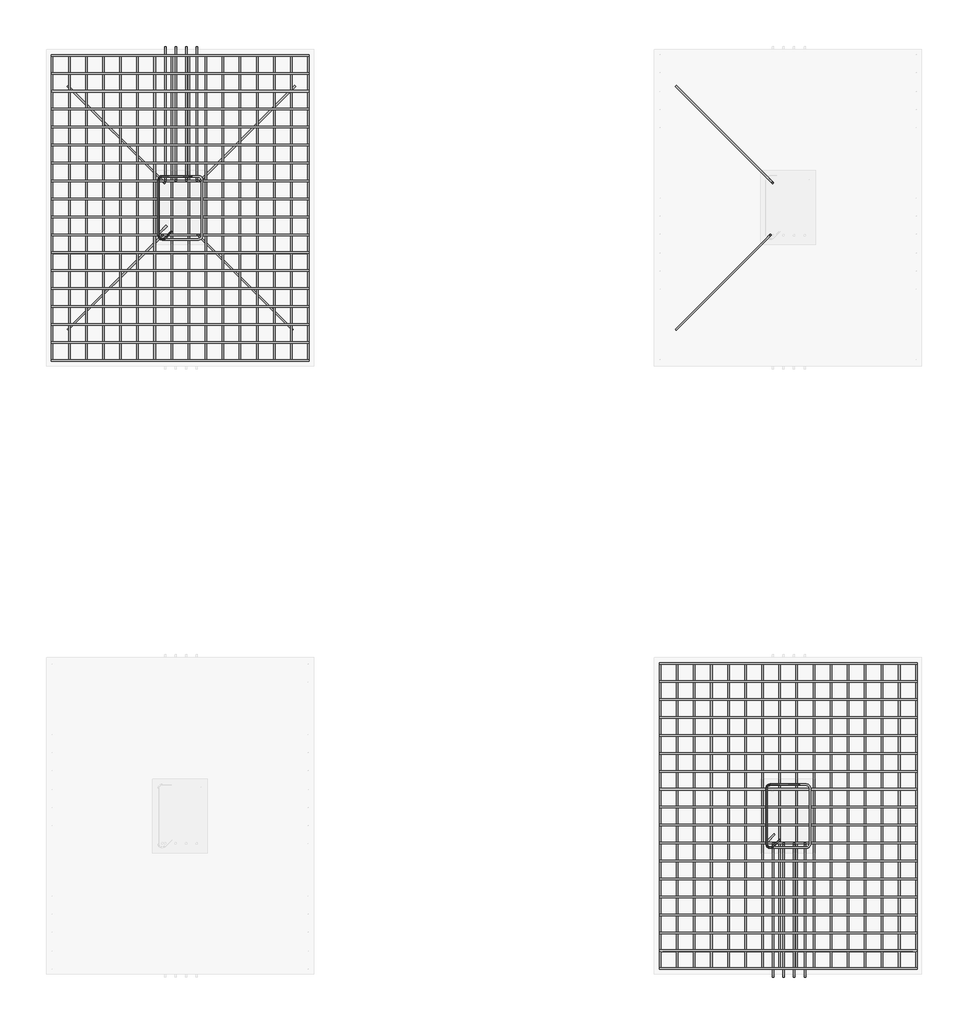
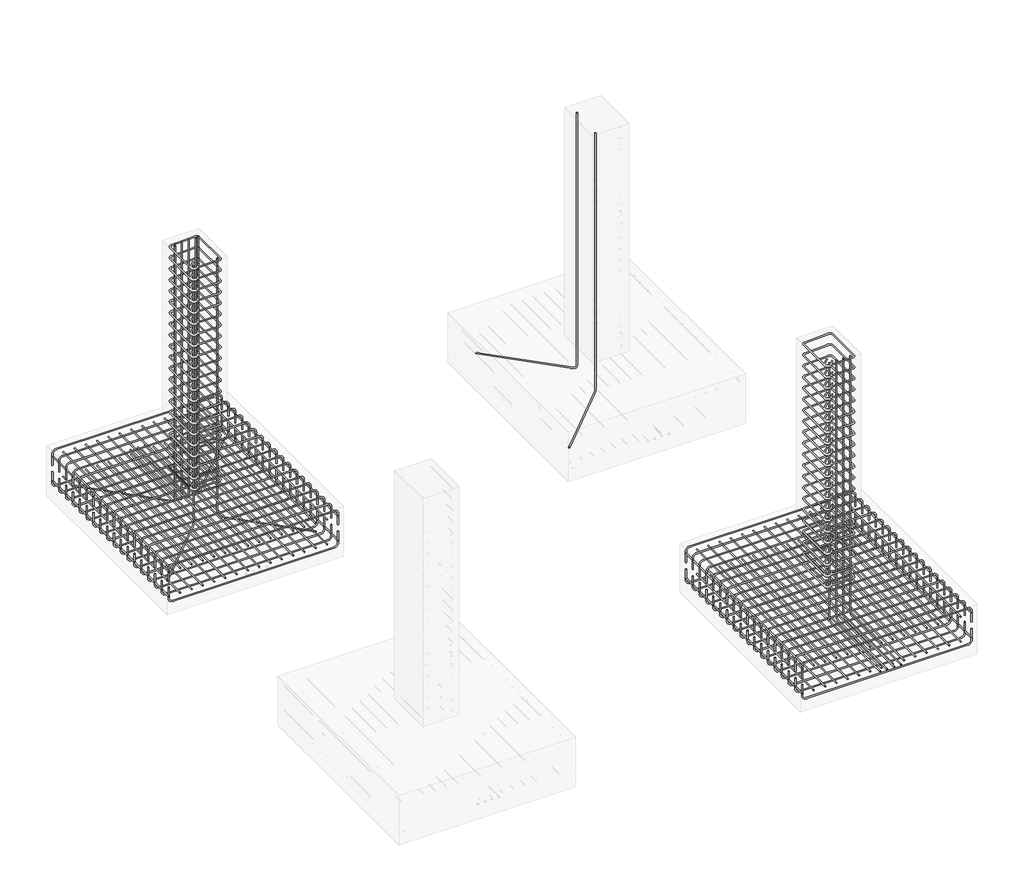
# One storey, part 6 of 33: 18 reinforcing bars.
"""IFC4 building model written with IfcOpenShell, lengths in millimetres."""

from ifc_helpers import new_model, si_unit, point, frame, origin, place, context, project, spatial, polyline, circle_curve, trimmed, segment, composite_curve, source, transform, mapped, element, save
from ifc_brep_helpers import swept_disk

model = new_model("IFC4")

# Units and contexts
model_context = context("Model", 3, world=origin())
ifc_project = project(units=[si_unit("LENGTHUNIT", "METRE", prefix="MILLI")], contexts=[model_context])

# Site, building, storey
site = spatial("IfcSite", under=ifc_project)
building = spatial("IfcBuilding", under=site)
storey = spatial("IfcBuildingStorey", under=building, Elevation=-3000.0)

# Reinforcing bars
placement = place(None, origin())
reinforcing_bar_shape = source(origin(), model_context, "Body", "SolidModel", [
    swept_disk(composite_curve([segment(polyline([(-693.4642742, -7044.0608134, -3240.0), (-693.4642742, -7044.0608134, -3092.7)]), True, "CONTINUOUS"), segment(trimmed(circle_curve(frame((-647.1142742, -7044.0608134, -3092.7), z_axis=(0.0, 1.0, 0.0), x_axis=(-46.35000000000002, 0.0, 0.0)), 46.35), [point((-693.4642742, -7044.0608134, -3092.7))], [point((-647.1142742, -7044.0608134, -3046.35))], True, "CARTESIAN"), True, "CONTINUOUS"), segment(polyline([(-647.1142742, -7044.0608134, -3046.35), (1367.4857258, -7044.0608134, -3046.35)]), True, "CONTINUOUS"), segment(trimmed(circle_curve(frame((1367.4857258, -7044.0608134, -3092.7), z_axis=(0.0, 1.0, 0.0), x_axis=(0.0, 0.0, 46.34999999999991)), 46.35), [point((1367.4857258, -7044.0608134, -3046.35))], [point((1413.8357258, -7044.0608134, -3092.7))], True, "CARTESIAN"), True, "CONTINUOUS"), segment(polyline([(1413.8357258, -7044.0608134, -3092.7), (1413.8357258, -7044.0608134, -3240.0)]), True, "CONTINUOUS")], self_intersect=False), 6.35),
])
element("IfcReinforcingBar", 1, at=placement, inside=storey, context=model_context, shape_type="MappedRepresentation", body=[
    mapped(reinforcing_bar_shape, transform((0.0, 0.0, 0.0), x_axis=(1.0, 0.0, 0.0), y_axis=(0.0, 1.0, 0.0), z_axis=(0.0, 0.0, 1.0))),
    mapped(reinforcing_bar_shape, transform((0.0, -147.4882353, 0.0), x_axis=(1.0, 0.0, 0.0), y_axis=(0.0, 1.0, 0.0), z_axis=(0.0, 0.0, 1.0))),
    mapped(reinforcing_bar_shape, transform((0.0, -294.9764706, 0.0), x_axis=(1.0, 0.0, 0.0), y_axis=(0.0, 1.0, 0.0), z_axis=(0.0, 0.0, 1.0))),
    mapped(reinforcing_bar_shape, transform((0.0, -442.4647059, 0.0), x_axis=(1.0, 0.0, 0.0), y_axis=(0.0, 1.0, 0.0), z_axis=(0.0, 0.0, 1.0))),
    mapped(reinforcing_bar_shape, transform((0.0, -589.9529412, 0.0), x_axis=(1.0, 0.0, 0.0), y_axis=(0.0, 1.0, 0.0), z_axis=(0.0, 0.0, 1.0))),
    mapped(reinforcing_bar_shape, transform((0.0, -737.4411765, 0.0), x_axis=(1.0, 0.0, 0.0), y_axis=(0.0, 1.0, 0.0), z_axis=(0.0, 0.0, 1.0))),
    mapped(reinforcing_bar_shape, transform((0.0, -884.9294118, 0.0), x_axis=(1.0, 0.0, 0.0), y_axis=(0.0, 1.0, 0.0), z_axis=(0.0, 0.0, 1.0))),
    mapped(reinforcing_bar_shape, transform((0.0, -1032.4176471, 0.0), x_axis=(1.0, 0.0, 0.0), y_axis=(0.0, 1.0, 0.0), z_axis=(0.0, 0.0, 1.0))),
    mapped(reinforcing_bar_shape, transform((0.0, -1179.9058824, 0.0), x_axis=(1.0, 0.0, 0.0), y_axis=(0.0, 1.0, 0.0), z_axis=(0.0, 0.0, 1.0))),
    mapped(reinforcing_bar_shape, transform((0.0, -1327.3941176, 0.0), x_axis=(1.0, 0.0, 0.0), y_axis=(0.0, 1.0, 0.0), z_axis=(0.0, 0.0, 1.0))),
    mapped(reinforcing_bar_shape, transform((0.0, -1474.8823529, 0.0), x_axis=(1.0, 0.0, 0.0), y_axis=(0.0, 1.0, 0.0), z_axis=(0.0, 0.0, 1.0))),
    mapped(reinforcing_bar_shape, transform((0.0, -1622.3705882, 0.0), x_axis=(1.0, 0.0, 0.0), y_axis=(0.0, 1.0, 0.0), z_axis=(0.0, 0.0, 1.0))),
    mapped(reinforcing_bar_shape, transform((0.0, -1769.8588235, 0.0), x_axis=(1.0, 0.0, 0.0), y_axis=(0.0, 1.0, 0.0), z_axis=(0.0, 0.0, 1.0))),
    mapped(reinforcing_bar_shape, transform((0.0, -1917.3470588, 0.0), x_axis=(1.0, 0.0, 0.0), y_axis=(0.0, 1.0, 0.0), z_axis=(0.0, 0.0, 1.0))),
    mapped(reinforcing_bar_shape, transform((0.0, -2064.8352941, 0.0), x_axis=(1.0, 0.0, 0.0), y_axis=(0.0, 1.0, 0.0), z_axis=(0.0, 0.0, 1.0))),
    mapped(reinforcing_bar_shape, transform((0.0, -2212.3235294, 0.0), x_axis=(1.0, 0.0, 0.0), y_axis=(0.0, 1.0, 0.0), z_axis=(0.0, 0.0, 1.0))),
    mapped(reinforcing_bar_shape, transform((0.0, -2359.8117647, 0.0), x_axis=(1.0, 0.0, 0.0), y_axis=(0.0, 1.0, 0.0), z_axis=(0.0, 0.0, 1.0))),
    mapped(reinforcing_bar_shape, transform((0.0, -2507.3, 0.0), x_axis=(1.0, 0.0, 0.0), y_axis=(0.0, 1.0, 0.0), z_axis=(0.0, 0.0, 1.0))),
])
reinforcing_bar_2_shape = source(origin(), model_context, "Body", "SolidModel", [
    swept_disk(composite_curve([segment(polyline([(1413.8357258, -7044.0608134, -3330.080452), (1413.8357258, -7044.0608134, -3477.380452)]), True, "CONTINUOUS"), segment(trimmed(circle_curve(frame((1367.4857258, -7044.0608134, -3477.380452), z_axis=(0.0, 1.0, 0.0), x_axis=(46.350000000000136, 0.0, 0.0)), 46.35), [point((1413.8357258, -7044.0608134, -3477.380452))], [point((1367.4857258, -7044.0608134, -3523.730452))], True, "CARTESIAN"), True, "CONTINUOUS"), segment(polyline([(1367.4857258, -7044.0608134, -3523.730452), (-647.1142742, -7044.0608134, -3523.730452)]), True, "CONTINUOUS"), segment(trimmed(circle_curve(frame((-647.1142742, -7044.0608134, -3477.380452), z_axis=(0.0, 1.0, 0.0), x_axis=(0.0, 0.0, -46.34999999999991)), 46.35), [point((-647.1142742, -7044.0608134, -3523.730452))], [point((-693.4642742, -7044.0608134, -3477.380452))], True, "CARTESIAN"), True, "CONTINUOUS"), segment(polyline([(-693.4642742, -7044.0608134, -3477.380452), (-693.4642742, -7044.0608134, -3330.080452)]), True, "CONTINUOUS")], self_intersect=False), 6.35),
])
element("IfcReinforcingBar", 2, at=placement, inside=storey, context=model_context, shape_type="MappedRepresentation", body=[
    mapped(reinforcing_bar_2_shape, transform((0.0, 0.0, 0.0), x_axis=(1.0, 0.0, 0.0), y_axis=(0.0, 1.0, 0.0), z_axis=(0.0, 0.0, 1.0))),
    mapped(reinforcing_bar_2_shape, transform((0.0, -147.4882353, 0.0), x_axis=(1.0, 0.0, 0.0), y_axis=(0.0, 1.0, 0.0), z_axis=(0.0, 0.0, 1.0))),
    mapped(reinforcing_bar_2_shape, transform((0.0, -294.9764706, 0.0), x_axis=(1.0, 0.0, 0.0), y_axis=(0.0, 1.0, 0.0), z_axis=(0.0, 0.0, 1.0))),
    mapped(reinforcing_bar_2_shape, transform((0.0, -442.4647059, 0.0), x_axis=(1.0, 0.0, 0.0), y_axis=(0.0, 1.0, 0.0), z_axis=(0.0, 0.0, 1.0))),
    mapped(reinforcing_bar_2_shape, transform((0.0, -589.9529412, 0.0), x_axis=(1.0, 0.0, 0.0), y_axis=(0.0, 1.0, 0.0), z_axis=(0.0, 0.0, 1.0))),
    mapped(reinforcing_bar_2_shape, transform((0.0, -737.4411765, 0.0), x_axis=(1.0, 0.0, 0.0), y_axis=(0.0, 1.0, 0.0), z_axis=(0.0, 0.0, 1.0))),
    mapped(reinforcing_bar_2_shape, transform((0.0, -884.9294118, 0.0), x_axis=(1.0, 0.0, 0.0), y_axis=(0.0, 1.0, 0.0), z_axis=(0.0, 0.0, 1.0))),
    mapped(reinforcing_bar_2_shape, transform((0.0, -1032.4176471, 0.0), x_axis=(1.0, 0.0, 0.0), y_axis=(0.0, 1.0, 0.0), z_axis=(0.0, 0.0, 1.0))),
    mapped(reinforcing_bar_2_shape, transform((0.0, -1179.9058824, 0.0), x_axis=(1.0, 0.0, 0.0), y_axis=(0.0, 1.0, 0.0), z_axis=(0.0, 0.0, 1.0))),
    mapped(reinforcing_bar_2_shape, transform((0.0, -1327.3941176, 0.0), x_axis=(1.0, 0.0, 0.0), y_axis=(0.0, 1.0, 0.0), z_axis=(0.0, 0.0, 1.0))),
    mapped(reinforcing_bar_2_shape, transform((0.0, -1474.8823529, 0.0), x_axis=(1.0, 0.0, 0.0), y_axis=(0.0, 1.0, 0.0), z_axis=(0.0, 0.0, 1.0))),
    mapped(reinforcing_bar_2_shape, transform((0.0, -1622.3705882, 0.0), x_axis=(1.0, 0.0, 0.0), y_axis=(0.0, 1.0, 0.0), z_axis=(0.0, 0.0, 1.0))),
    mapped(reinforcing_bar_2_shape, transform((0.0, -1769.8588235, 0.0), x_axis=(1.0, 0.0, 0.0), y_axis=(0.0, 1.0, 0.0), z_axis=(0.0, 0.0, 1.0))),
    mapped(reinforcing_bar_2_shape, transform((0.0, -1917.3470588, 0.0), x_axis=(1.0, 0.0, 0.0), y_axis=(0.0, 1.0, 0.0), z_axis=(0.0, 0.0, 1.0))),
    mapped(reinforcing_bar_2_shape, transform((0.0, -2064.8352941, 0.0), x_axis=(1.0, 0.0, 0.0), y_axis=(0.0, 1.0, 0.0), z_axis=(0.0, 0.0, 1.0))),
    mapped(reinforcing_bar_2_shape, transform((0.0, -2212.3235294, 0.0), x_axis=(1.0, 0.0, 0.0), y_axis=(0.0, 1.0, 0.0), z_axis=(0.0, 0.0, 1.0))),
    mapped(reinforcing_bar_2_shape, transform((0.0, -2359.8117647, 0.0), x_axis=(1.0, 0.0, 0.0), y_axis=(0.0, 1.0, 0.0), z_axis=(0.0, 0.0, 1.0))),
    mapped(reinforcing_bar_2_shape, transform((0.0, -2507.3, 0.0), x_axis=(1.0, 0.0, 0.0), y_axis=(0.0, 1.0, 0.0), z_axis=(0.0, 0.0, 1.0))),
])
reinforcing_bar_3_shape = source(origin(), model_context, "Body", "SolidModel", [
    swept_disk(composite_curve([segment(polyline([(1413.8357258, -9557.7108134, -3447.8614173), (1413.8357258, -7037.7108134, -3447.8614173)]), True, "CONTINUOUS")], self_intersect=False), 6.35),
])
element("IfcReinforcingBar", 3, at=placement, inside=storey, context=model_context, shape_type="MappedRepresentation", body=[
    mapped(reinforcing_bar_3_shape, transform((0.0, 0.0, 0.0), x_axis=(1.0, 0.0, 0.0), y_axis=(0.0, 1.0, 0.0), z_axis=(0.0, 0.0, 1.0))),
    mapped(reinforcing_bar_3_shape, transform((-140.4866667, 0.0, 0.0), x_axis=(1.0, 0.0, 0.0), y_axis=(0.0, 1.0, 0.0), z_axis=(0.0, 0.0, 1.0))),
    mapped(reinforcing_bar_3_shape, transform((-280.9733333, 0.0, 0.0), x_axis=(1.0, 0.0, 0.0), y_axis=(0.0, 1.0, 0.0), z_axis=(0.0, 0.0, 1.0))),
    mapped(reinforcing_bar_3_shape, transform((-421.46, 0.0, 0.0), x_axis=(1.0, 0.0, 0.0), y_axis=(0.0, 1.0, 0.0), z_axis=(0.0, 0.0, 1.0))),
    mapped(reinforcing_bar_3_shape, transform((-561.9466667, 0.0, 0.0), x_axis=(1.0, 0.0, 0.0), y_axis=(0.0, 1.0, 0.0), z_axis=(0.0, 0.0, 1.0))),
    mapped(reinforcing_bar_3_shape, transform((-702.4333333, 0.0, 0.0), x_axis=(1.0, 0.0, 0.0), y_axis=(0.0, 1.0, 0.0), z_axis=(0.0, 0.0, 1.0))),
    mapped(reinforcing_bar_3_shape, transform((-842.92, 0.0, 0.0), x_axis=(1.0, 0.0, 0.0), y_axis=(0.0, 1.0, 0.0), z_axis=(0.0, 0.0, 1.0))),
    mapped(reinforcing_bar_3_shape, transform((-983.4066667, 0.0, 0.0), x_axis=(1.0, 0.0, 0.0), y_axis=(0.0, 1.0, 0.0), z_axis=(0.0, 0.0, 1.0))),
    mapped(reinforcing_bar_3_shape, transform((-1123.8933333, 0.0, 0.0), x_axis=(1.0, 0.0, 0.0), y_axis=(0.0, 1.0, 0.0), z_axis=(0.0, 0.0, 1.0))),
    mapped(reinforcing_bar_3_shape, transform((-1264.38, 0.0, 0.0), x_axis=(1.0, 0.0, 0.0), y_axis=(0.0, 1.0, 0.0), z_axis=(0.0, 0.0, 1.0))),
    mapped(reinforcing_bar_3_shape, transform((-1404.8666667, 0.0, 0.0), x_axis=(1.0, 0.0, 0.0), y_axis=(0.0, 1.0, 0.0), z_axis=(0.0, 0.0, 1.0))),
    mapped(reinforcing_bar_3_shape, transform((-1545.3533333, 0.0, 0.0), x_axis=(1.0, 0.0, 0.0), y_axis=(0.0, 1.0, 0.0), z_axis=(0.0, 0.0, 1.0))),
    mapped(reinforcing_bar_3_shape, transform((-1685.84, 0.0, 0.0), x_axis=(1.0, 0.0, 0.0), y_axis=(0.0, 1.0, 0.0), z_axis=(0.0, 0.0, 1.0))),
    mapped(reinforcing_bar_3_shape, transform((-1826.3266667, 0.0, 0.0), x_axis=(1.0, 0.0, 0.0), y_axis=(0.0, 1.0, 0.0), z_axis=(0.0, 0.0, 1.0))),
    mapped(reinforcing_bar_3_shape, transform((-1966.8133333, 0.0, 0.0), x_axis=(1.0, 0.0, 0.0), y_axis=(0.0, 1.0, 0.0), z_axis=(0.0, 0.0, 1.0))),
    mapped(reinforcing_bar_3_shape, transform((-2107.3, 0.0, 0.0), x_axis=(1.0, 0.0, 0.0), y_axis=(0.0, 1.0, 0.0), z_axis=(0.0, 0.0, 1.0))),
])
reinforcing_bar_4_shape = source(origin(), model_context, "Body", "SolidModel", [
    swept_disk(composite_curve([segment(polyline([(-693.4642742, -9557.7108134, -3122.7084113), (-693.4642742, -7037.7108134, -3122.7084113)]), True, "CONTINUOUS")], self_intersect=False), 6.35),
])
element("IfcReinforcingBar", 4, at=placement, inside=storey, context=model_context, shape_type="MappedRepresentation", body=[
    mapped(reinforcing_bar_4_shape, transform((0.0, 0.0, 0.0), x_axis=(1.0, 0.0, 0.0), y_axis=(0.0, 1.0, 0.0), z_axis=(0.0, 0.0, 1.0))),
    mapped(reinforcing_bar_4_shape, transform((140.4866667, 0.0, 0.0), x_axis=(1.0, 0.0, 0.0), y_axis=(0.0, 1.0, 0.0), z_axis=(0.0, 0.0, 1.0))),
    mapped(reinforcing_bar_4_shape, transform((280.9733333, 0.0, 0.0), x_axis=(1.0, 0.0, 0.0), y_axis=(0.0, 1.0, 0.0), z_axis=(0.0, 0.0, 1.0))),
    mapped(reinforcing_bar_4_shape, transform((421.46, 0.0, 0.0), x_axis=(1.0, 0.0, 0.0), y_axis=(0.0, 1.0, 0.0), z_axis=(0.0, 0.0, 1.0))),
    mapped(reinforcing_bar_4_shape, transform((561.9466667, 0.0, 0.0), x_axis=(1.0, 0.0, 0.0), y_axis=(0.0, 1.0, 0.0), z_axis=(0.0, 0.0, 1.0))),
    mapped(reinforcing_bar_4_shape, transform((702.4333333, 0.0, 0.0), x_axis=(1.0, 0.0, 0.0), y_axis=(0.0, 1.0, 0.0), z_axis=(0.0, 0.0, 1.0))),
    mapped(reinforcing_bar_4_shape, transform((842.92, 0.0, 0.0), x_axis=(1.0, 0.0, 0.0), y_axis=(0.0, 1.0, 0.0), z_axis=(0.0, 0.0, 1.0))),
    mapped(reinforcing_bar_4_shape, transform((983.4066667, 0.0, 0.0), x_axis=(1.0, 0.0, 0.0), y_axis=(0.0, 1.0, 0.0), z_axis=(0.0, 0.0, 1.0))),
    mapped(reinforcing_bar_4_shape, transform((1123.8933333, 0.0, 0.0), x_axis=(1.0, 0.0, 0.0), y_axis=(0.0, 1.0, 0.0), z_axis=(0.0, 0.0, 1.0))),
    mapped(reinforcing_bar_4_shape, transform((1264.38, 0.0, 0.0), x_axis=(1.0, 0.0, 0.0), y_axis=(0.0, 1.0, 0.0), z_axis=(0.0, 0.0, 1.0))),
    mapped(reinforcing_bar_4_shape, transform((1404.8666667, 0.0, 0.0), x_axis=(1.0, 0.0, 0.0), y_axis=(0.0, 1.0, 0.0), z_axis=(0.0, 0.0, 1.0))),
    mapped(reinforcing_bar_4_shape, transform((1545.3533333, 0.0, 0.0), x_axis=(1.0, 0.0, 0.0), y_axis=(0.0, 1.0, 0.0), z_axis=(0.0, 0.0, 1.0))),
    mapped(reinforcing_bar_4_shape, transform((1685.84, 0.0, 0.0), x_axis=(1.0, 0.0, 0.0), y_axis=(0.0, 1.0, 0.0), z_axis=(0.0, 0.0, 1.0))),
    mapped(reinforcing_bar_4_shape, transform((1826.3266667, 0.0, 0.0), x_axis=(1.0, 0.0, 0.0), y_axis=(0.0, 1.0, 0.0), z_axis=(0.0, 0.0, 1.0))),
    mapped(reinforcing_bar_4_shape, transform((1966.8133333, 0.0, 0.0), x_axis=(1.0, 0.0, 0.0), y_axis=(0.0, 1.0, 0.0), z_axis=(0.0, 0.0, 1.0))),
    mapped(reinforcing_bar_4_shape, transform((2107.3, 0.0, 0.0), x_axis=(1.0, 0.0, 0.0), y_axis=(0.0, 1.0, 0.0), z_axis=(0.0, 0.0, 1.0))),
])
reinforcing_bar_5_shape = source(origin(), model_context, "Body", "SolidModel", [
    swept_disk(composite_curve([segment(polyline([(-5693.4642742, -2044.0608134, -3240.0), (-5693.4642742, -2044.0608134, -3092.7)]), True, "CONTINUOUS"), segment(trimmed(circle_curve(frame((-5647.1142742, -2044.0608134, -3092.7), z_axis=(0.0, 1.0, 0.0), x_axis=(-46.349999999999454, 0.0, 0.0)), 46.35), [point((-5693.4642742, -2044.0608134, -3092.7))], [point((-5647.1142742, -2044.0608134, -3046.35))], True, "CARTESIAN"), True, "CONTINUOUS"), segment(polyline([(-5647.1142742, -2044.0608134, -3046.35), (-3632.5142742, -2044.0608134, -3046.35)]), True, "CONTINUOUS"), segment(trimmed(circle_curve(frame((-3632.5142742, -2044.0608134, -3092.7), z_axis=(0.0, 1.0, 0.0), x_axis=(0.0, 0.0, 46.34999999999991)), 46.35), [point((-3632.5142742, -2044.0608134, -3046.35))], [point((-3586.1642742, -2044.0608134, -3092.7))], True, "CARTESIAN"), True, "CONTINUOUS"), segment(polyline([(-3586.1642742, -2044.0608134, -3092.7), (-3586.1642742, -2044.0608134, -3240.0)]), True, "CONTINUOUS")], self_intersect=False), 6.35),
])
element("IfcReinforcingBar", 5, at=placement, inside=storey, context=model_context, shape_type="MappedRepresentation", body=[
    mapped(reinforcing_bar_5_shape, transform((0.0, 0.0, 0.0), x_axis=(1.0, 0.0, 0.0), y_axis=(0.0, 1.0, 0.0), z_axis=(0.0, 0.0, 1.0))),
    mapped(reinforcing_bar_5_shape, transform((0.0, -147.4882353, 0.0), x_axis=(1.0, 0.0, 0.0), y_axis=(0.0, 1.0, 0.0), z_axis=(0.0, 0.0, 1.0))),
    mapped(reinforcing_bar_5_shape, transform((0.0, -294.9764706, 0.0), x_axis=(1.0, 0.0, 0.0), y_axis=(0.0, 1.0, 0.0), z_axis=(0.0, 0.0, 1.0))),
    mapped(reinforcing_bar_5_shape, transform((0.0, -442.4647059, 0.0), x_axis=(1.0, 0.0, 0.0), y_axis=(0.0, 1.0, 0.0), z_axis=(0.0, 0.0, 1.0))),
    mapped(reinforcing_bar_5_shape, transform((0.0, -589.9529412, 0.0), x_axis=(1.0, 0.0, 0.0), y_axis=(0.0, 1.0, 0.0), z_axis=(0.0, 0.0, 1.0))),
    mapped(reinforcing_bar_5_shape, transform((0.0, -737.4411765, 0.0), x_axis=(1.0, 0.0, 0.0), y_axis=(0.0, 1.0, 0.0), z_axis=(0.0, 0.0, 1.0))),
    mapped(reinforcing_bar_5_shape, transform((0.0, -884.9294118, 0.0), x_axis=(1.0, 0.0, 0.0), y_axis=(0.0, 1.0, 0.0), z_axis=(0.0, 0.0, 1.0))),
    mapped(reinforcing_bar_5_shape, transform((0.0, -1032.4176471, 0.0), x_axis=(1.0, 0.0, 0.0), y_axis=(0.0, 1.0, 0.0), z_axis=(0.0, 0.0, 1.0))),
    mapped(reinforcing_bar_5_shape, transform((0.0, -1179.9058824, 0.0), x_axis=(1.0, 0.0, 0.0), y_axis=(0.0, 1.0, 0.0), z_axis=(0.0, 0.0, 1.0))),
    mapped(reinforcing_bar_5_shape, transform((0.0, -1327.3941176, 0.0), x_axis=(1.0, 0.0, 0.0), y_axis=(0.0, 1.0, 0.0), z_axis=(0.0, 0.0, 1.0))),
    mapped(reinforcing_bar_5_shape, transform((0.0, -1474.8823529, 0.0), x_axis=(1.0, 0.0, 0.0), y_axis=(0.0, 1.0, 0.0), z_axis=(0.0, 0.0, 1.0))),
    mapped(reinforcing_bar_5_shape, transform((0.0, -1622.3705882, 0.0), x_axis=(1.0, 0.0, 0.0), y_axis=(0.0, 1.0, 0.0), z_axis=(0.0, 0.0, 1.0))),
    mapped(reinforcing_bar_5_shape, transform((0.0, -1769.8588235, 0.0), x_axis=(1.0, 0.0, 0.0), y_axis=(0.0, 1.0, 0.0), z_axis=(0.0, 0.0, 1.0))),
    mapped(reinforcing_bar_5_shape, transform((0.0, -1917.3470588, 0.0), x_axis=(1.0, 0.0, 0.0), y_axis=(0.0, 1.0, 0.0), z_axis=(0.0, 0.0, 1.0))),
    mapped(reinforcing_bar_5_shape, transform((0.0, -2064.8352941, 0.0), x_axis=(1.0, 0.0, 0.0), y_axis=(0.0, 1.0, 0.0), z_axis=(0.0, 0.0, 1.0))),
    mapped(reinforcing_bar_5_shape, transform((0.0, -2212.3235294, 0.0), x_axis=(1.0, 0.0, 0.0), y_axis=(0.0, 1.0, 0.0), z_axis=(0.0, 0.0, 1.0))),
    mapped(reinforcing_bar_5_shape, transform((0.0, -2359.8117647, 0.0), x_axis=(1.0, 0.0, 0.0), y_axis=(0.0, 1.0, 0.0), z_axis=(0.0, 0.0, 1.0))),
    mapped(reinforcing_bar_5_shape, transform((0.0, -2507.3, 0.0), x_axis=(1.0, 0.0, 0.0), y_axis=(0.0, 1.0, 0.0), z_axis=(0.0, 0.0, 1.0))),
])
reinforcing_bar_6_shape = source(origin(), model_context, "Body", "SolidModel", [
    swept_disk(composite_curve([segment(polyline([(-3586.1642742, -2044.0608134, -3330.080452), (-3586.1642742, -2044.0608134, -3477.380452)]), True, "CONTINUOUS"), segment(trimmed(circle_curve(frame((-3632.5142742, -2044.0608134, -3477.380452), z_axis=(0.0, 1.0, 0.0), x_axis=(46.34999999999991, 0.0, 0.0)), 46.35), [point((-3586.1642742, -2044.0608134, -3477.380452))], [point((-3632.5142742, -2044.0608134, -3523.730452))], True, "CARTESIAN"), True, "CONTINUOUS"), segment(polyline([(-3632.5142742, -2044.0608134, -3523.730452), (-5647.1142742, -2044.0608134, -3523.730452)]), True, "CONTINUOUS"), segment(trimmed(circle_curve(frame((-5647.1142742, -2044.0608134, -3477.380452), z_axis=(0.0, 1.0, 0.0), x_axis=(0.0, 0.0, -46.34999999999991)), 46.35), [point((-5647.1142742, -2044.0608134, -3523.730452))], [point((-5693.4642742, -2044.0608134, -3477.380452))], True, "CARTESIAN"), True, "CONTINUOUS"), segment(polyline([(-5693.4642742, -2044.0608134, -3477.380452), (-5693.4642742, -2044.0608134, -3330.080452)]), True, "CONTINUOUS")], self_intersect=False), 6.35),
])
element("IfcReinforcingBar", 6, at=placement, inside=storey, context=model_context, shape_type="MappedRepresentation", body=[
    mapped(reinforcing_bar_6_shape, transform((0.0, 0.0, 0.0), x_axis=(1.0, 0.0, 0.0), y_axis=(0.0, 1.0, 0.0), z_axis=(0.0, 0.0, 1.0))),
    mapped(reinforcing_bar_6_shape, transform((0.0, -147.4882353, 0.0), x_axis=(1.0, 0.0, 0.0), y_axis=(0.0, 1.0, 0.0), z_axis=(0.0, 0.0, 1.0))),
    mapped(reinforcing_bar_6_shape, transform((0.0, -294.9764706, 0.0), x_axis=(1.0, 0.0, 0.0), y_axis=(0.0, 1.0, 0.0), z_axis=(0.0, 0.0, 1.0))),
    mapped(reinforcing_bar_6_shape, transform((0.0, -442.4647059, 0.0), x_axis=(1.0, 0.0, 0.0), y_axis=(0.0, 1.0, 0.0), z_axis=(0.0, 0.0, 1.0))),
    mapped(reinforcing_bar_6_shape, transform((0.0, -589.9529412, 0.0), x_axis=(1.0, 0.0, 0.0), y_axis=(0.0, 1.0, 0.0), z_axis=(0.0, 0.0, 1.0))),
    mapped(reinforcing_bar_6_shape, transform((0.0, -737.4411765, 0.0), x_axis=(1.0, 0.0, 0.0), y_axis=(0.0, 1.0, 0.0), z_axis=(0.0, 0.0, 1.0))),
    mapped(reinforcing_bar_6_shape, transform((0.0, -884.9294118, 0.0), x_axis=(1.0, 0.0, 0.0), y_axis=(0.0, 1.0, 0.0), z_axis=(0.0, 0.0, 1.0))),
    mapped(reinforcing_bar_6_shape, transform((0.0, -1032.4176471, 0.0), x_axis=(1.0, 0.0, 0.0), y_axis=(0.0, 1.0, 0.0), z_axis=(0.0, 0.0, 1.0))),
    mapped(reinforcing_bar_6_shape, transform((0.0, -1179.9058824, 0.0), x_axis=(1.0, 0.0, 0.0), y_axis=(0.0, 1.0, 0.0), z_axis=(0.0, 0.0, 1.0))),
    mapped(reinforcing_bar_6_shape, transform((0.0, -1327.3941176, 0.0), x_axis=(1.0, 0.0, 0.0), y_axis=(0.0, 1.0, 0.0), z_axis=(0.0, 0.0, 1.0))),
    mapped(reinforcing_bar_6_shape, transform((0.0, -1474.8823529, 0.0), x_axis=(1.0, 0.0, 0.0), y_axis=(0.0, 1.0, 0.0), z_axis=(0.0, 0.0, 1.0))),
    mapped(reinforcing_bar_6_shape, transform((0.0, -1622.3705882, 0.0), x_axis=(1.0, 0.0, 0.0), y_axis=(0.0, 1.0, 0.0), z_axis=(0.0, 0.0, 1.0))),
    mapped(reinforcing_bar_6_shape, transform((0.0, -1769.8588235, 0.0), x_axis=(1.0, 0.0, 0.0), y_axis=(0.0, 1.0, 0.0), z_axis=(0.0, 0.0, 1.0))),
    mapped(reinforcing_bar_6_shape, transform((0.0, -1917.3470588, 0.0), x_axis=(1.0, 0.0, 0.0), y_axis=(0.0, 1.0, 0.0), z_axis=(0.0, 0.0, 1.0))),
    mapped(reinforcing_bar_6_shape, transform((0.0, -2064.8352941, 0.0), x_axis=(1.0, 0.0, 0.0), y_axis=(0.0, 1.0, 0.0), z_axis=(0.0, 0.0, 1.0))),
    mapped(reinforcing_bar_6_shape, transform((0.0, -2212.3235294, 0.0), x_axis=(1.0, 0.0, 0.0), y_axis=(0.0, 1.0, 0.0), z_axis=(0.0, 0.0, 1.0))),
    mapped(reinforcing_bar_6_shape, transform((0.0, -2359.8117647, 0.0), x_axis=(1.0, 0.0, 0.0), y_axis=(0.0, 1.0, 0.0), z_axis=(0.0, 0.0, 1.0))),
    mapped(reinforcing_bar_6_shape, transform((0.0, -2507.3, 0.0), x_axis=(1.0, 0.0, 0.0), y_axis=(0.0, 1.0, 0.0), z_axis=(0.0, 0.0, 1.0))),
])
reinforcing_bar_7_shape = source(origin(), model_context, "Body", "SolidModel", [
    swept_disk(composite_curve([segment(polyline([(-3586.1642742, -4557.7108134, -3447.8614173), (-3586.1642742, -2037.7108134, -3447.8614173)]), True, "CONTINUOUS")], self_intersect=False), 6.35),
])
element("IfcReinforcingBar", 7, at=placement, inside=storey, context=model_context, shape_type="MappedRepresentation", body=[
    mapped(reinforcing_bar_7_shape, transform((0.0, 0.0, 0.0), x_axis=(1.0, 0.0, 0.0), y_axis=(0.0, 1.0, 0.0), z_axis=(0.0, 0.0, 1.0))),
    mapped(reinforcing_bar_7_shape, transform((-140.4866667, 0.0, 0.0), x_axis=(1.0, 0.0, 0.0), y_axis=(0.0, 1.0, 0.0), z_axis=(0.0, 0.0, 1.0))),
    mapped(reinforcing_bar_7_shape, transform((-280.9733333, 0.0, 0.0), x_axis=(1.0, 0.0, 0.0), y_axis=(0.0, 1.0, 0.0), z_axis=(0.0, 0.0, 1.0))),
    mapped(reinforcing_bar_7_shape, transform((-421.46, 0.0, 0.0), x_axis=(1.0, 0.0, 0.0), y_axis=(0.0, 1.0, 0.0), z_axis=(0.0, 0.0, 1.0))),
    mapped(reinforcing_bar_7_shape, transform((-561.9466667, 0.0, 0.0), x_axis=(1.0, 0.0, 0.0), y_axis=(0.0, 1.0, 0.0), z_axis=(0.0, 0.0, 1.0))),
    mapped(reinforcing_bar_7_shape, transform((-702.4333333, 0.0, 0.0), x_axis=(1.0, 0.0, 0.0), y_axis=(0.0, 1.0, 0.0), z_axis=(0.0, 0.0, 1.0))),
    mapped(reinforcing_bar_7_shape, transform((-842.92, 0.0, 0.0), x_axis=(1.0, 0.0, 0.0), y_axis=(0.0, 1.0, 0.0), z_axis=(0.0, 0.0, 1.0))),
    mapped(reinforcing_bar_7_shape, transform((-983.4066667, 0.0, 0.0), x_axis=(1.0, 0.0, 0.0), y_axis=(0.0, 1.0, 0.0), z_axis=(0.0, 0.0, 1.0))),
    mapped(reinforcing_bar_7_shape, transform((-1123.8933333, 0.0, 0.0), x_axis=(1.0, 0.0, 0.0), y_axis=(0.0, 1.0, 0.0), z_axis=(0.0, 0.0, 1.0))),
    mapped(reinforcing_bar_7_shape, transform((-1264.38, 0.0, 0.0), x_axis=(1.0, 0.0, 0.0), y_axis=(0.0, 1.0, 0.0), z_axis=(0.0, 0.0, 1.0))),
    mapped(reinforcing_bar_7_shape, transform((-1404.8666667, 0.0, 0.0), x_axis=(1.0, 0.0, 0.0), y_axis=(0.0, 1.0, 0.0), z_axis=(0.0, 0.0, 1.0))),
    mapped(reinforcing_bar_7_shape, transform((-1545.3533333, 0.0, 0.0), x_axis=(1.0, 0.0, 0.0), y_axis=(0.0, 1.0, 0.0), z_axis=(0.0, 0.0, 1.0))),
    mapped(reinforcing_bar_7_shape, transform((-1685.84, 0.0, 0.0), x_axis=(1.0, 0.0, 0.0), y_axis=(0.0, 1.0, 0.0), z_axis=(0.0, 0.0, 1.0))),
    mapped(reinforcing_bar_7_shape, transform((-1826.3266667, 0.0, 0.0), x_axis=(1.0, 0.0, 0.0), y_axis=(0.0, 1.0, 0.0), z_axis=(0.0, 0.0, 1.0))),
    mapped(reinforcing_bar_7_shape, transform((-1966.8133333, 0.0, 0.0), x_axis=(1.0, 0.0, 0.0), y_axis=(0.0, 1.0, 0.0), z_axis=(0.0, 0.0, 1.0))),
    mapped(reinforcing_bar_7_shape, transform((-2107.3, 0.0, 0.0), x_axis=(1.0, 0.0, 0.0), y_axis=(0.0, 1.0, 0.0), z_axis=(0.0, 0.0, 1.0))),
])
reinforcing_bar_8_shape = source(origin(), model_context, "Body", "SolidModel", [
    swept_disk(composite_curve([segment(polyline([(-5693.4642742, -4557.7108134, -3122.7084113), (-5693.4642742, -2037.7108134, -3122.7084113)]), True, "CONTINUOUS")], self_intersect=False), 6.35),
])
element("IfcReinforcingBar", 8, at=placement, inside=storey, context=model_context, shape_type="MappedRepresentation", body=[
    mapped(reinforcing_bar_8_shape, transform((0.0, 0.0, 0.0), x_axis=(1.0, 0.0, 0.0), y_axis=(0.0, 1.0, 0.0), z_axis=(0.0, 0.0, 1.0))),
    mapped(reinforcing_bar_8_shape, transform((140.4866667, 0.0, 0.0), x_axis=(1.0, 0.0, 0.0), y_axis=(0.0, 1.0, 0.0), z_axis=(0.0, 0.0, 1.0))),
    mapped(reinforcing_bar_8_shape, transform((280.9733333, 0.0, 0.0), x_axis=(1.0, 0.0, 0.0), y_axis=(0.0, 1.0, 0.0), z_axis=(0.0, 0.0, 1.0))),
    mapped(reinforcing_bar_8_shape, transform((421.46, 0.0, 0.0), x_axis=(1.0, 0.0, 0.0), y_axis=(0.0, 1.0, 0.0), z_axis=(0.0, 0.0, 1.0))),
    mapped(reinforcing_bar_8_shape, transform((561.9466667, 0.0, 0.0), x_axis=(1.0, 0.0, 0.0), y_axis=(0.0, 1.0, 0.0), z_axis=(0.0, 0.0, 1.0))),
    mapped(reinforcing_bar_8_shape, transform((702.4333333, 0.0, 0.0), x_axis=(1.0, 0.0, 0.0), y_axis=(0.0, 1.0, 0.0), z_axis=(0.0, 0.0, 1.0))),
    mapped(reinforcing_bar_8_shape, transform((842.92, 0.0, 0.0), x_axis=(1.0, 0.0, 0.0), y_axis=(0.0, 1.0, 0.0), z_axis=(0.0, 0.0, 1.0))),
    mapped(reinforcing_bar_8_shape, transform((983.4066667, 0.0, 0.0), x_axis=(1.0, 0.0, 0.0), y_axis=(0.0, 1.0, 0.0), z_axis=(0.0, 0.0, 1.0))),
    mapped(reinforcing_bar_8_shape, transform((1123.8933333, 0.0, 0.0), x_axis=(1.0, 0.0, 0.0), y_axis=(0.0, 1.0, 0.0), z_axis=(0.0, 0.0, 1.0))),
    mapped(reinforcing_bar_8_shape, transform((1264.38, 0.0, 0.0), x_axis=(1.0, 0.0, 0.0), y_axis=(0.0, 1.0, 0.0), z_axis=(0.0, 0.0, 1.0))),
    mapped(reinforcing_bar_8_shape, transform((1404.8666667, 0.0, 0.0), x_axis=(1.0, 0.0, 0.0), y_axis=(0.0, 1.0, 0.0), z_axis=(0.0, 0.0, 1.0))),
    mapped(reinforcing_bar_8_shape, transform((1545.3533333, 0.0, 0.0), x_axis=(1.0, 0.0, 0.0), y_axis=(0.0, 1.0, 0.0), z_axis=(0.0, 0.0, 1.0))),
    mapped(reinforcing_bar_8_shape, transform((1685.84, 0.0, 0.0), x_axis=(1.0, 0.0, 0.0), y_axis=(0.0, 1.0, 0.0), z_axis=(0.0, 0.0, 1.0))),
    mapped(reinforcing_bar_8_shape, transform((1826.3266667, 0.0, 0.0), x_axis=(1.0, 0.0, 0.0), y_axis=(0.0, 1.0, 0.0), z_axis=(0.0, 0.0, 1.0))),
    mapped(reinforcing_bar_8_shape, transform((1966.8133333, 0.0, 0.0), x_axis=(1.0, 0.0, 0.0), y_axis=(0.0, 1.0, 0.0), z_axis=(0.0, 0.0, 1.0))),
    mapped(reinforcing_bar_8_shape, transform((2107.3, 0.0, 0.0), x_axis=(1.0, 0.0, 0.0), y_axis=(0.0, 1.0, 0.0), z_axis=(0.0, 0.0, 1.0))),
])
reinforcing_bar_9_shape = source(origin(), model_context, "Body", "SolidModel", [
    swept_disk(composite_curve([segment(polyline([(-4753.5385089, -3446.8994528, -2953.65), (-4809.2820718, -3502.6430158, -2953.65)]), True, "CONTINUOUS"), segment(trimmed(circle_curve(frame((-4787.1142742, -3524.8108134, -2953.65), z_axis=(0.0, 0.0, 1.0), x_axis=(-22.167797600000085, 22.167797600000085, 0.0)), 31.35), [point((-4809.2820718, -3502.6430158, -2953.65))], [point((-4787.1142742, -3556.1608134, -2953.65))], True, "CARTESIAN"), True, "CONTINUOUS"), segment(polyline([(-4787.1142742, -3556.1608134, -2953.65), (-4492.5142742, -3556.1608134, -2953.65)]), True, "CONTINUOUS"), segment(trimmed(circle_curve(frame((-4492.5142742, -3524.8108134, -2953.65), z_axis=(0.0, 0.0, 1.0), x_axis=(0.0, -31.34999999999991, 0.0)), 31.35), [point((-4492.5142742, -3556.1608134, -2953.65))], [point((-4461.1642742, -3524.8108134, -2953.65))], True, "CARTESIAN"), True, "CONTINUOUS"), segment(polyline([(-4461.1642742, -3524.8108134, -2953.65), (-4461.1642742, -3070.6108134, -2953.65)]), True, "CONTINUOUS"), segment(trimmed(circle_curve(frame((-4492.4944891, -3070.6108134, -2954.7636125), z_axis=(-0.0355219283344822, 0.0, 0.9993688971583016), x_axis=(31.33021489999919, 0.0, 1.1136124999998174)), 31.35), [point((-4461.1642742, -3070.6108134, -2953.65))], [point((-4492.4944891, -3039.2608134, -2954.7636125))], True, "CARTESIAN"), True, "CONTINUOUS"), segment(polyline([(-4492.4944891, -3039.2608134, -2954.7636125), (-4787.1340593, -3039.2608134, -2965.2363875)]), True, "CONTINUOUS"), segment(trimmed(circle_curve(frame((-4787.1340593, -3070.6108134, -2965.2363875), z_axis=(-0.0355219283344822, 0.0, 0.9993688971583016), x_axis=(0.0, 31.34999999999991, 0.0)), 31.35), [point((-4787.1340593, -3039.2608134, -2965.2363875))], [point((-4818.4642742, -3070.6108134, -2966.35))], True, "CARTESIAN"), True, "CONTINUOUS"), segment(polyline([(-4818.4642742, -3070.6108134, -2966.35), (-4818.4642742, -3524.8108134, -2966.35)]), True, "CONTINUOUS"), segment(trimmed(circle_curve(frame((-4787.1142742, -3524.8108134, -2966.35), z_axis=(0.0, 0.0, 1.0), x_axis=(-31.349999999999454, 0.0, 0.0)), 31.35), [point((-4818.4642742, -3524.8108134, -2966.35))], [point((-4764.9464766, -3546.978611, -2966.35))], True, "CARTESIAN"), True, "CONTINUOUS"), segment(polyline([(-4764.9464766, -3546.978611, -2966.35), (-4709.2029137, -3491.235048, -2966.35)]), True, "CONTINUOUS")], self_intersect=False), 6.35),
])
element("IfcReinforcingBar", 9, at=placement, inside=storey, context=model_context, shape_type="MappedRepresentation", body=[
    mapped(reinforcing_bar_9_shape, transform((0.0, 0.0, 0.0), x_axis=(1.0, 0.0, 0.0), y_axis=(0.0, 1.0, 0.0), z_axis=(0.0, 0.0, 1.0))),
    mapped(reinforcing_bar_9_shape, transform((0.0, 0.0, 145.365), x_axis=(1.0, 0.0, 0.0), y_axis=(0.0, 1.0, 0.0), z_axis=(0.0, 0.0, 1.0))),
    mapped(reinforcing_bar_9_shape, transform((0.0, 0.0, 290.73), x_axis=(1.0, 0.0, 0.0), y_axis=(0.0, 1.0, 0.0), z_axis=(0.0, 0.0, 1.0))),
    mapped(reinforcing_bar_9_shape, transform((0.0, 0.0, 436.095), x_axis=(1.0, 0.0, 0.0), y_axis=(0.0, 1.0, 0.0), z_axis=(0.0, 0.0, 1.0))),
    mapped(reinforcing_bar_9_shape, transform((0.0, 0.0, 581.46), x_axis=(1.0, 0.0, 0.0), y_axis=(0.0, 1.0, 0.0), z_axis=(0.0, 0.0, 1.0))),
    mapped(reinforcing_bar_9_shape, transform((0.0, 0.0, 726.825), x_axis=(1.0, 0.0, 0.0), y_axis=(0.0, 1.0, 0.0), z_axis=(0.0, 0.0, 1.0))),
    mapped(reinforcing_bar_9_shape, transform((0.0, 0.0, 872.19), x_axis=(1.0, 0.0, 0.0), y_axis=(0.0, 1.0, 0.0), z_axis=(0.0, 0.0, 1.0))),
    mapped(reinforcing_bar_9_shape, transform((0.0, 0.0, 1017.555), x_axis=(1.0, 0.0, 0.0), y_axis=(0.0, 1.0, 0.0), z_axis=(0.0, 0.0, 1.0))),
    mapped(reinforcing_bar_9_shape, transform((0.0, 0.0, 1162.92), x_axis=(1.0, 0.0, 0.0), y_axis=(0.0, 1.0, 0.0), z_axis=(0.0, 0.0, 1.0))),
    mapped(reinforcing_bar_9_shape, transform((0.0, 0.0, 1308.285), x_axis=(1.0, 0.0, 0.0), y_axis=(0.0, 1.0, 0.0), z_axis=(0.0, 0.0, 1.0))),
    mapped(reinforcing_bar_9_shape, transform((0.0, 0.0, 1453.65), x_axis=(1.0, 0.0, 0.0), y_axis=(0.0, 1.0, 0.0), z_axis=(0.0, 0.0, 1.0))),
    mapped(reinforcing_bar_9_shape, transform((0.0, 0.0, 1599.015), x_axis=(1.0, 0.0, 0.0), y_axis=(0.0, 1.0, 0.0), z_axis=(0.0, 0.0, 1.0))),
    mapped(reinforcing_bar_9_shape, transform((0.0, 0.0, 1744.38), x_axis=(1.0, 0.0, 0.0), y_axis=(0.0, 1.0, 0.0), z_axis=(0.0, 0.0, 1.0))),
    mapped(reinforcing_bar_9_shape, transform((0.0, 0.0, 1889.745), x_axis=(1.0, 0.0, 0.0), y_axis=(0.0, 1.0, 0.0), z_axis=(0.0, 0.0, 1.0))),
    mapped(reinforcing_bar_9_shape, transform((0.0, 0.0, 2035.11), x_axis=(1.0, 0.0, 0.0), y_axis=(0.0, 1.0, 0.0), z_axis=(0.0, 0.0, 1.0))),
    mapped(reinforcing_bar_9_shape, transform((0.0, 0.0, 2180.475), x_axis=(1.0, 0.0, 0.0), y_axis=(0.0, 1.0, 0.0), z_axis=(0.0, 0.0, 1.0))),
    mapped(reinforcing_bar_9_shape, transform((0.0, 0.0, 2325.84), x_axis=(1.0, 0.0, 0.0), y_axis=(0.0, 1.0, 0.0), z_axis=(0.0, 0.0, 1.0))),
    mapped(reinforcing_bar_9_shape, transform((0.0, 0.0, 2471.205), x_axis=(1.0, 0.0, 0.0), y_axis=(0.0, 1.0, 0.0), z_axis=(0.0, 0.0, 1.0))),
    mapped(reinforcing_bar_9_shape, transform((0.0, 0.0, 2616.57), x_axis=(1.0, 0.0, 0.0), y_axis=(0.0, 1.0, 0.0), z_axis=(0.0, 0.0, 1.0))),
    mapped(reinforcing_bar_9_shape, transform((0.0, 0.0, 2761.935), x_axis=(1.0, 0.0, 0.0), y_axis=(0.0, 1.0, 0.0), z_axis=(0.0, 0.0, 1.0))),
    mapped(reinforcing_bar_9_shape, transform((0.0, 0.0, 2907.3), x_axis=(1.0, 0.0, 0.0), y_axis=(0.0, 1.0, 0.0), z_axis=(0.0, 0.0, 1.0))),
])
element("IfcReinforcingBar", 10, at=placement, inside=storey, context=model_context, shape_type="SolidModel", body=[
    swept_disk(composite_curve([segment(polyline([(-4786.7956786, -3521.6339414, -40.0), (-4786.7956786, -3521.6339414, -3393.65)]), True, "CONTINUOUS"), segment(trimmed(circle_curve(frame((-4819.5700779, -3554.4083407, -3393.65), z_axis=(-0.7071067811865446, 0.7071067811865505, 0.0), x_axis=(32.77439929999946, 32.774399299999914, 0.0)), 46.35), [point((-4786.7956786, -3521.6339414, -3393.65))], [point((-4819.5700779, -3554.4083407, -3440.0))], True, "CARTESIAN"), True, "CONTINUOUS"), segment(polyline([(-4819.5700779, -3554.4083407, -3440.0), (-5564.6131379, -4299.4514007, -3440.0)]), True, "CONTINUOUS")], self_intersect=False), 6.35),
])
element("IfcReinforcingBar", 11, at=placement, inside=storey, context=model_context, shape_type="SolidModel", body=[
    swept_disk(composite_curve([segment(polyline([(-4768.8975726, -3091.6857913, -40.0), (-4768.8975726, -3091.6857913, -3361.434517)]), True, "CONTINUOUS"), segment(trimmed(circle_curve(frame((-4801.6719719, -3058.911392, -3361.434517), z_axis=(0.7071067811865539, 0.7071067811865411, 0.0), x_axis=(32.77439930000037, -32.774399299999914, 0.0)), 46.35), [point((-4768.8975726, -3091.6857913, -3361.434517))], [point((-4801.6719719, -3058.911392, -3407.784517))], True, "CARTESIAN"), True, "CONTINUOUS"), segment(polyline([(-4801.6719719, -3058.911392, -3407.784517), (-5564.6131379, -2295.970226, -3407.784517)]), True, "CONTINUOUS")], self_intersect=False), 6.35),
])
element("IfcReinforcingBar", 12, at=placement, inside=storey, context=model_context, shape_type="SolidModel", body=[
    swept_disk(composite_curve([segment(polyline([(-4492.8328699, -3521.6339414, -40.0), (-4492.8328699, -3521.6339414, -3393.65)]), True, "CONTINUOUS"), segment(trimmed(circle_curve(frame((-4460.0584706, -3554.4083407, -3393.65), z_axis=(-0.7071067811865493, -0.7071067811865459, 0.0), x_axis=(-32.77439930000037, 32.774399299999914, 0.0)), 46.35), [point((-4492.8328699, -3521.6339414, -3393.65))], [point((-4460.0584706, -3554.4083407, -3440.0))], True, "CARTESIAN"), True, "CONTINUOUS"), segment(polyline([(-4460.0584706, -3554.4083407, -3440.0), (-3715.0154106, -4299.4514007, -3440.0)]), True, "CONTINUOUS")], self_intersect=False), 6.35),
])
element("IfcReinforcingBar", 13, at=placement, inside=storey, context=model_context, shape_type="SolidModel", body=[
    swept_disk(composite_curve([segment(polyline([(-4474.2315783, -3073.7876853, -30.2564663), (-4474.2315783, -3073.7876853, -3383.9064663)]), True, "CONTINUOUS"), segment(trimmed(circle_curve(frame((-4441.457179, -3041.013286, -3383.9064663), z_axis=(0.7071067811865493, -0.7071067811865459, 0.0), x_axis=(-32.77439930000037, -32.774399299999914, 0.0)), 46.35), [point((-4474.2315783, -3073.7876853, -3383.9064663))], [point((-4441.457179, -3041.013286, -3430.2564663))], True, "CARTESIAN"), True, "CONTINUOUS"), segment(polyline([(-4441.457179, -3041.013286, -3430.2564663), (-3696.414119, -2295.970226, -3430.2564663)]), True, "CONTINUOUS")], self_intersect=False), 6.35),
])
reinforcing_bar_10_shape = source(origin(), model_context, "Body", "SolidModel", [
    swept_disk(composite_curve([segment(polyline([(-4763.8841678, -3071.9278134, -40.0), (-4763.8841678, -3071.9278134, -3393.65)]), True, "CONTINUOUS"), segment(trimmed(circle_curve(frame((-4763.8841678, -3025.5778134, -3393.65), z_axis=(1.0, 0.0, 0.0), x_axis=(0.0, -46.34999999999991, 0.0)), 46.35), [point((-4763.8841678, -3071.9278134, -3393.65))], [point((-4763.8841678, -3025.5778134, -3440.0))], True, "CARTESIAN"), True, "CONTINUOUS"), segment(polyline([(-4763.8841678, -3025.5778134, -3440.0), (-4763.8841678, -1971.9278134, -3440.0)]), True, "CONTINUOUS")], self_intersect=False), 6.35),
])
element("IfcReinforcingBar", 14, at=placement, inside=storey, context=model_context, shape_type="MappedRepresentation", body=[
    mapped(reinforcing_bar_10_shape, transform((0.0, 0.0, 0.0), x_axis=(1.0, 0.0, 0.0), y_axis=(0.0, 1.0, 0.0), z_axis=(0.0, 0.0, 1.0))),
    mapped(reinforcing_bar_10_shape, transform((86.8979716, 0.0, 0.0), x_axis=(1.0, 0.0, 0.0), y_axis=(0.0, 1.0, 0.0), z_axis=(0.0, 0.0, 1.0))),
    mapped(reinforcing_bar_10_shape, transform((173.7959432, 0.0, 0.0), x_axis=(1.0, 0.0, 0.0), y_axis=(0.0, 1.0, 0.0), z_axis=(0.0, 0.0, 1.0))),
    mapped(reinforcing_bar_10_shape, transform((260.6939148, 0.0, 0.0), x_axis=(1.0, 0.0, 0.0), y_axis=(0.0, 1.0, 0.0), z_axis=(0.0, 0.0, 1.0))),
])
element("IfcReinforcingBar", 15, at=placement, inside=storey, context=model_context, shape_type="SolidModel", body=[
    swept_disk(composite_curve([segment(polyline([(213.2043214, -3521.6339414, -40.0), (213.2043214, -3521.6339414, -3393.65)]), True, "CONTINUOUS"), segment(trimmed(circle_curve(frame((180.4299221, -3554.4083407, -3393.65), z_axis=(-0.7071067811865446, 0.7071067811865505, 0.0), x_axis=(32.7743993, 32.774399299999914, 0.0)), 46.35), [point((213.2043214, -3521.6339414, -3393.65))], [point((180.4299221, -3554.4083407, -3440.0))], True, "CARTESIAN"), True, "CONTINUOUS"), segment(polyline([(180.4299221, -3554.4083407, -3440.0), (-564.6131379, -4299.4514007, -3440.0)]), True, "CONTINUOUS")], self_intersect=False), 6.35),
])
element("IfcReinforcingBar", 16, at=placement, inside=storey, context=model_context, shape_type="SolidModel", body=[
    swept_disk(composite_curve([segment(polyline([(231.1024274, -3091.6857913, -40.0), (231.1024274, -3091.6857913, -3361.434517)]), True, "CONTINUOUS"), segment(trimmed(circle_curve(frame((198.3280281, -3058.911392, -3361.434517), z_axis=(0.7071067811865539, 0.7071067811865411, 0.0), x_axis=(32.7743993, -32.774399299999914, 0.0)), 46.35), [point((231.1024274, -3091.6857913, -3361.434517))], [point((198.3280281, -3058.911392, -3407.784517))], True, "CARTESIAN"), True, "CONTINUOUS"), segment(polyline([(198.3280281, -3058.911392, -3407.784517), (-564.6131379, -2295.970226, -3407.784517)]), True, "CONTINUOUS")], self_intersect=False), 6.35),
])
reinforcing_bar_11_shape = source(origin(), model_context, "Body", "SolidModel", [
    swept_disk(composite_curve([segment(polyline([(246.4614911, -8446.8994528, -2953.65), (190.7179282, -8502.6430158, -2953.65)]), True, "CONTINUOUS"), segment(trimmed(circle_curve(frame((212.8857258, -8524.8108134, -2953.65), z_axis=(0.0, 0.0, 1.0), x_axis=(-22.1677976, 22.167797599999176, 0.0)), 31.35), [point((190.7179282, -8502.6430158, -2953.65))], [point((212.8857258, -8556.1608134, -2953.65))], True, "CARTESIAN"), True, "CONTINUOUS"), segment(polyline([(212.8857258, -8556.1608134, -2953.65), (507.4857258, -8556.1608134, -2953.65)]), True, "CONTINUOUS"), segment(trimmed(circle_curve(frame((507.4857258, -8524.8108134, -2953.65), z_axis=(0.0, 0.0, 1.0), x_axis=(0.0, -31.350000000000364, 0.0)), 31.35), [point((507.4857258, -8556.1608134, -2953.65))], [point((538.8357258, -8524.8108134, -2953.65))], True, "CARTESIAN"), True, "CONTINUOUS"), segment(polyline([(538.8357258, -8524.8108134, -2953.65), (538.8357258, -8070.6108134, -2953.65)]), True, "CONTINUOUS"), segment(trimmed(circle_curve(frame((507.5055109, -8070.6108134, -2954.7636125), z_axis=(-0.0355219283344822, 0.0, 0.9993688971583016), x_axis=(31.330214899999987, 0.0, 1.1136124999998174)), 31.35), [point((538.8357258, -8070.6108134, -2953.65))], [point((507.5055109, -8039.2608134, -2954.7636125))], True, "CARTESIAN"), True, "CONTINUOUS"), segment(polyline([(507.5055109, -8039.2608134, -2954.7636125), (212.8659407, -8039.2608134, -2965.2363875)]), True, "CONTINUOUS"), segment(trimmed(circle_curve(frame((212.8659407, -8070.6108134, -2965.2363875), z_axis=(-0.0355219283344822, 0.0, 0.9993688971583016), x_axis=(0.0, 31.349999999999454, 0.0)), 31.35), [point((212.8659407, -8039.2608134, -2965.2363875))], [point((181.5357258, -8070.6108134, -2966.35))], True, "CARTESIAN"), True, "CONTINUOUS"), segment(polyline([(181.5357258, -8070.6108134, -2966.35), (181.5357258, -8524.8108134, -2966.35)]), True, "CONTINUOUS"), segment(trimmed(circle_curve(frame((212.8857258, -8524.8108134, -2966.35), z_axis=(0.0, 0.0, 1.0), x_axis=(-31.349999999999994, 0.0, 0.0)), 31.35), [point((181.5357258, -8524.8108134, -2966.35))], [point((235.0535234, -8546.978611, -2966.35))], True, "CARTESIAN"), True, "CONTINUOUS"), segment(polyline([(235.0535234, -8546.978611, -2966.35), (290.7970863, -8491.235048, -2966.35)]), True, "CONTINUOUS")], self_intersect=False), 6.35),
])
element("IfcReinforcingBar", 17, at=placement, inside=storey, context=model_context, shape_type="MappedRepresentation", body=[
    mapped(reinforcing_bar_11_shape, transform((0.0, 0.0, 0.0), x_axis=(1.0, 0.0, 0.0), y_axis=(0.0, 1.0, 0.0), z_axis=(0.0, 0.0, 1.0))),
    mapped(reinforcing_bar_11_shape, transform((0.0, 0.0, 145.365), x_axis=(1.0, 0.0, 0.0), y_axis=(0.0, 1.0, 0.0), z_axis=(0.0, 0.0, 1.0))),
    mapped(reinforcing_bar_11_shape, transform((0.0, 0.0, 290.73), x_axis=(1.0, 0.0, 0.0), y_axis=(0.0, 1.0, 0.0), z_axis=(0.0, 0.0, 1.0))),
    mapped(reinforcing_bar_11_shape, transform((0.0, 0.0, 436.095), x_axis=(1.0, 0.0, 0.0), y_axis=(0.0, 1.0, 0.0), z_axis=(0.0, 0.0, 1.0))),
    mapped(reinforcing_bar_11_shape, transform((0.0, 0.0, 581.46), x_axis=(1.0, 0.0, 0.0), y_axis=(0.0, 1.0, 0.0), z_axis=(0.0, 0.0, 1.0))),
    mapped(reinforcing_bar_11_shape, transform((0.0, 0.0, 726.825), x_axis=(1.0, 0.0, 0.0), y_axis=(0.0, 1.0, 0.0), z_axis=(0.0, 0.0, 1.0))),
    mapped(reinforcing_bar_11_shape, transform((0.0, 0.0, 872.19), x_axis=(1.0, 0.0, 0.0), y_axis=(0.0, 1.0, 0.0), z_axis=(0.0, 0.0, 1.0))),
    mapped(reinforcing_bar_11_shape, transform((0.0, 0.0, 1017.555), x_axis=(1.0, 0.0, 0.0), y_axis=(0.0, 1.0, 0.0), z_axis=(0.0, 0.0, 1.0))),
    mapped(reinforcing_bar_11_shape, transform((0.0, 0.0, 1162.92), x_axis=(1.0, 0.0, 0.0), y_axis=(0.0, 1.0, 0.0), z_axis=(0.0, 0.0, 1.0))),
    mapped(reinforcing_bar_11_shape, transform((0.0, 0.0, 1308.285), x_axis=(1.0, 0.0, 0.0), y_axis=(0.0, 1.0, 0.0), z_axis=(0.0, 0.0, 1.0))),
    mapped(reinforcing_bar_11_shape, transform((0.0, 0.0, 1453.65), x_axis=(1.0, 0.0, 0.0), y_axis=(0.0, 1.0, 0.0), z_axis=(0.0, 0.0, 1.0))),
    mapped(reinforcing_bar_11_shape, transform((0.0, 0.0, 1599.015), x_axis=(1.0, 0.0, 0.0), y_axis=(0.0, 1.0, 0.0), z_axis=(0.0, 0.0, 1.0))),
    mapped(reinforcing_bar_11_shape, transform((0.0, 0.0, 1744.38), x_axis=(1.0, 0.0, 0.0), y_axis=(0.0, 1.0, 0.0), z_axis=(0.0, 0.0, 1.0))),
    mapped(reinforcing_bar_11_shape, transform((0.0, 0.0, 1889.745), x_axis=(1.0, 0.0, 0.0), y_axis=(0.0, 1.0, 0.0), z_axis=(0.0, 0.0, 1.0))),
    mapped(reinforcing_bar_11_shape, transform((0.0, 0.0, 2035.11), x_axis=(1.0, 0.0, 0.0), y_axis=(0.0, 1.0, 0.0), z_axis=(0.0, 0.0, 1.0))),
    mapped(reinforcing_bar_11_shape, transform((0.0, 0.0, 2180.475), x_axis=(1.0, 0.0, 0.0), y_axis=(0.0, 1.0, 0.0), z_axis=(0.0, 0.0, 1.0))),
    mapped(reinforcing_bar_11_shape, transform((0.0, 0.0, 2325.84), x_axis=(1.0, 0.0, 0.0), y_axis=(0.0, 1.0, 0.0), z_axis=(0.0, 0.0, 1.0))),
    mapped(reinforcing_bar_11_shape, transform((0.0, 0.0, 2471.205), x_axis=(1.0, 0.0, 0.0), y_axis=(0.0, 1.0, 0.0), z_axis=(0.0, 0.0, 1.0))),
    mapped(reinforcing_bar_11_shape, transform((0.0, 0.0, 2616.57), x_axis=(1.0, 0.0, 0.0), y_axis=(0.0, 1.0, 0.0), z_axis=(0.0, 0.0, 1.0))),
    mapped(reinforcing_bar_11_shape, transform((0.0, 0.0, 2761.935), x_axis=(1.0, 0.0, 0.0), y_axis=(0.0, 1.0, 0.0), z_axis=(0.0, 0.0, 1.0))),
    mapped(reinforcing_bar_11_shape, transform((0.0, 0.0, 2907.3), x_axis=(1.0, 0.0, 0.0), y_axis=(0.0, 1.0, 0.0), z_axis=(0.0, 0.0, 1.0))),
])
reinforcing_bar_12_shape = source(origin(), model_context, "Body", "SolidModel", [
    swept_disk(composite_curve([segment(polyline([(236.1158322, -8523.4938134, -40.0), (236.1158322, -8523.4938134, -3393.65)]), True, "CONTINUOUS"), segment(trimmed(circle_curve(frame((236.1158322, -8569.8438134, -3393.65), z_axis=(-1.0, 0.0, 0.0), x_axis=(0.0, 46.350000000000364, 0.0)), 46.35), [point((236.1158322, -8523.4938134, -3393.65))], [point((236.1158322, -8569.8438134, -3440.0))], True, "CARTESIAN"), True, "CONTINUOUS"), segment(polyline([(236.1158322, -8569.8438134, -3440.0), (236.1158322, -9623.4938134, -3440.0)]), True, "CONTINUOUS")], self_intersect=False), 6.35),
])
element("IfcReinforcingBar", 18, at=placement, inside=storey, context=model_context, shape_type="MappedRepresentation", body=[
    mapped(reinforcing_bar_12_shape, transform((0.0, 0.0, 0.0), x_axis=(1.0, 0.0, 0.0), y_axis=(0.0, 1.0, 0.0), z_axis=(0.0, 0.0, 1.0))),
    mapped(reinforcing_bar_12_shape, transform((86.8979716, 0.0, 0.0), x_axis=(1.0, 0.0, 0.0), y_axis=(0.0, 1.0, 0.0), z_axis=(0.0, 0.0, 1.0))),
    mapped(reinforcing_bar_12_shape, transform((173.7959432, 0.0, 0.0), x_axis=(1.0, 0.0, 0.0), y_axis=(0.0, 1.0, 0.0), z_axis=(0.0, 0.0, 1.0))),
    mapped(reinforcing_bar_12_shape, transform((260.6939148, 0.0, 0.0), x_axis=(1.0, 0.0, 0.0), y_axis=(0.0, 1.0, 0.0), z_axis=(0.0, 0.0, 1.0))),
])

save(model, "model.ifc")

# Revit data of these elements
# Elements 1, 2, 3, 4, 5, 6, 7, 8, 9, 10, 11, 12, 13, 14, 15, 16, 17, 18 (IfcReinforcingBar)
#   Phase Created = New Construction
